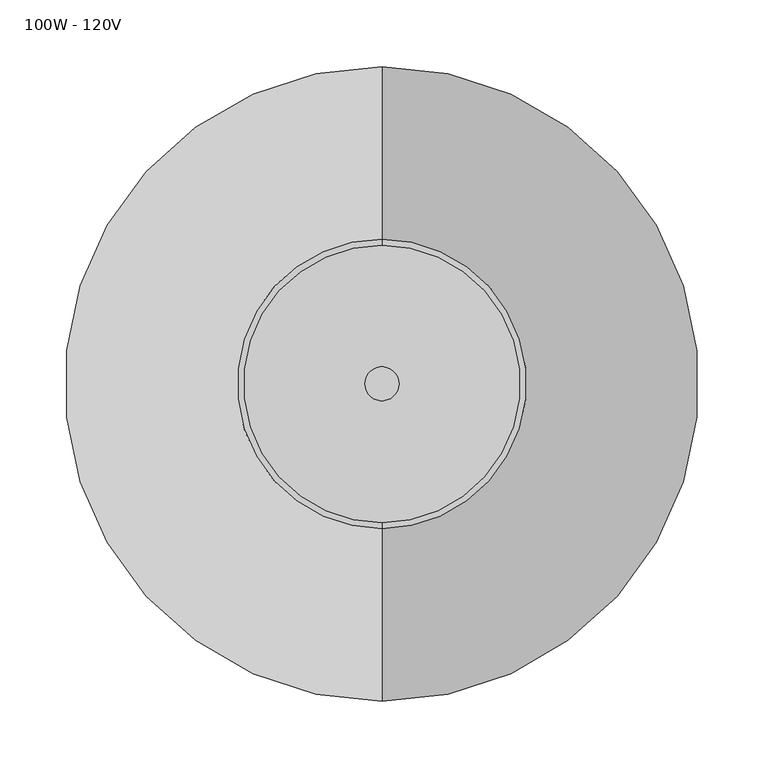
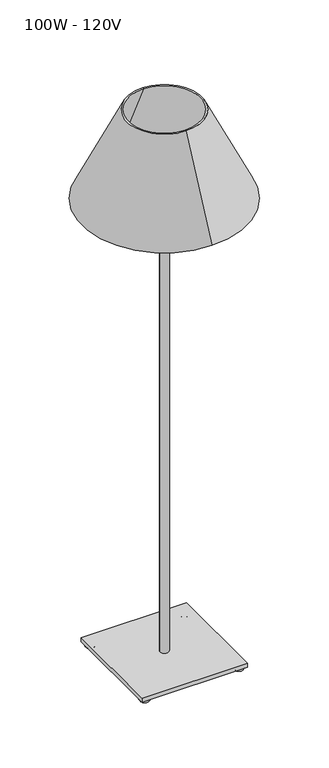
"""IFC4 building model written with IfcOpenShell, lengths in millimetres: light fixture geometry, 100W - 120V."""

from ifc_helpers import new_model, si_unit, point, frame, origin, origin_2d, place, context, project, spatial, polyline, circle_curve, ellipse_curve, trimmed, segment, composite_curve, outline, extrude, source, transform, mapped, element, save
from ifc_brep_helpers import plane_surface, revolved_surface, advanced_brep


def light_fixture_100w_120v_8564026f(model_context):
    return source(origin(), model_context, "Body", "SolidModel", [
        extrude(outline(composite_curve([segment(trimmed(circle_curve(origin_2d(), 12.7), [point((-12.7, 0.0))], [point((12.7, 0.0))], False, "CARTESIAN"), True, "CONTINUOUS"), segment(trimmed(circle_curve(origin_2d(), 12.7), [point((12.7, 0.0))], [point((-12.7, 0.0))], False, "CARTESIAN"), True, "CONTINUOUS")], self_intersect=False)), frame((0.0, 0.0, 24.9639672), z_axis=(0.0, 0.0, 1.0), x_axis=(1.0, 0.0, 0.0)), (0.0, 0.0, 1.0), 1499.0360328),
        extrude(outline(polyline([(152.4, 152.4), (152.4, -152.4), (-152.4, -152.4), (-152.4, 152.4), (152.4, 152.4)])), frame((0.0, 0.0, 12.6871384), z_axis=(0.0, 0.0, 1.0), x_axis=(1.0, 0.0, 0.0)), (0.0, 0.0, 1.0), 12.2768288),
        advanced_brep(
        [(133.9366871, -135.595774, 0.0), (140.1544999, -135.595774, 0.0), (140.1544999, -135.595774, 12.6871384), (133.9366871, -135.595774, 12.6871384), (121.2495488, -135.595774, 12.6871384), (152.8416383, -135.595774, 12.6871384)],
        [
            (0, 1, circle_curve(frame((137.0455935, -135.595774, 0.0), z_axis=(0.0, 0.0, -1.0), x_axis=(0.0, 1.0, 0.0)), 3.1089064)),
            (1, 2),
            (2, 3, circle_curve(frame((137.0455935, -135.595774, 12.6871384), z_axis=(0.0, 0.0, 1.0), x_axis=(0.0, 1.0, 0.0)), 3.1089064)),
            (3, 0),
            (1, 0, circle_curve(frame((137.0455935, -135.595774, 0.0), z_axis=(0.0, 0.0, -1.0), x_axis=(0.0, 1.0, 0.0)), 3.1089064)),
            (3, 2, circle_curve(frame((137.0455935, -135.595774, 12.6871384), z_axis=(0.0, 0.0, 1.0), x_axis=(0.0, 1.0, 0.0)), 3.1089064)),
            (4, 5, circle_curve(frame((137.0455935, -135.595774, 12.6871384), z_axis=(0.0, 0.0, -1.0), x_axis=(0.0, 1.0, 0.0)), 15.7960447)),
            (5, 1, circle_curve(frame((140.1544999, -135.595774, 12.6871384), z_axis=(0.0, 1.0, 0.0), x_axis=(1.0, 0.0, 0.0)), 12.6871384)),
            (0, 4, circle_curve(frame((133.9366871, -135.595774, 12.6871384), z_axis=(0.0, 1.0, 0.0), x_axis=(-1.0, 0.0, 0.0)), 12.6871384)),
            (5, 4, circle_curve(frame((137.0455935, -135.595774, 12.6871384), z_axis=(0.0, 0.0, -1.0), x_axis=(0.0, 1.0, 0.0)), 15.7960447)),
            (2, 5),
            (4, 3),
        ],
        [
            revolved_surface(polyline([(137.0455935, -132.4868676, 12.6871384), (137.0455935, -132.4868676, 0.0)]), (137.0455935, -135.595774, 0.0), (0.0, 0.0, 1.0)),
            revolved_surface(trimmed(ellipse_curve(frame((137.0455935, -132.4868676, 12.6871384), z_axis=(1.0, 0.0, 0.0), x_axis=(0.0, 1.0, 0.0)), 12.6871384, 12.6871384), [point((137.0455935, -132.4868676, 0.0))], [point((137.0455935, -119.7997292, 12.6871384))], True, "CARTESIAN"), (137.0455935, -135.595774, 0.0), (0.0, 0.0, 1.0)),
            plane_surface(frame((137.0455935, -135.595774, 12.6871384), z_axis=(0.0, 0.0, 1.0), x_axis=(0.0, 1.0, 0.0))),
        ],
        [
            (0, [[1, 2, 3, 4]]),
            (0, [[5, -4, 6, -2]]),
            (1, [[7, 8, -1, 9]]),
            (1, [[10, -9, -5, -8]]),
            (2, [[-3, 11, -7, 12]]),
            (2, [[-6, -12, -10, -11]]),
        ],
    ),
        advanced_brep(
        [(-138.5460372, -136.1907144, 0.0), (-132.3282244, -136.1907144, 0.0), (-132.3282244, -136.1907144, 12.6871384), (-138.5460372, -136.1907144, 12.6871384), (-151.2331755, -136.1907144, 12.6871384), (-119.641086, -136.1907144, 12.6871384)],
        [
            (0, 1, circle_curve(frame((-135.4371308, -136.1907144, 0.0), z_axis=(0.0, 0.0, -1.0), x_axis=(0.0, 1.0, 0.0)), 3.1089064)),
            (1, 2),
            (2, 3, circle_curve(frame((-135.4371308, -136.1907144, 12.6871384), z_axis=(0.0, 0.0, 1.0), x_axis=(0.0, 1.0, 0.0)), 3.1089064)),
            (3, 0),
            (1, 0, circle_curve(frame((-135.4371308, -136.1907144, 0.0), z_axis=(0.0, 0.0, -1.0), x_axis=(0.0, 1.0, 0.0)), 3.1089064)),
            (3, 2, circle_curve(frame((-135.4371308, -136.1907144, 12.6871384), z_axis=(0.0, 0.0, 1.0), x_axis=(0.0, 1.0, 0.0)), 3.1089064)),
            (4, 5, circle_curve(frame((-135.4371308, -136.1907144, 12.6871384), z_axis=(0.0, 0.0, -1.0), x_axis=(0.0, 1.0, 0.0)), 15.7960447)),
            (5, 1, circle_curve(frame((-132.3282244, -136.1907144, 12.6871384), z_axis=(0.0, 1.0, 0.0), x_axis=(1.0, 0.0, 0.0)), 12.6871384)),
            (0, 4, circle_curve(frame((-138.5460372, -136.1907144, 12.6871384), z_axis=(0.0, 1.0, 0.0), x_axis=(-1.0, 0.0, 0.0)), 12.6871384)),
            (5, 4, circle_curve(frame((-135.4371308, -136.1907144, 12.6871384), z_axis=(0.0, 0.0, -1.0), x_axis=(0.0, 1.0, 0.0)), 15.7960447)),
            (2, 5),
            (4, 3),
        ],
        [
            revolved_surface(polyline([(-135.4371308, -133.081808, 12.6871384), (-135.4371308, -133.081808, 0.0)]), (-135.4371308, -136.1907144, 0.0), (0.0, 0.0, 1.0)),
            revolved_surface(trimmed(ellipse_curve(frame((-135.4371308, -133.081808, 12.6871384), z_axis=(1.0, 0.0, 0.0), x_axis=(0.0, 1.0, 0.0)), 12.6871384, 12.6871384), [point((-135.4371308, -133.081808, 0.0))], [point((-135.4371308, -120.3946697, 12.6871384))], True, "CARTESIAN"), (-135.4371308, -136.1907144, 0.0), (0.0, 0.0, 1.0)),
            plane_surface(frame((-135.4371308, -136.1907144, 12.6871384), z_axis=(0.0, 0.0, 1.0), x_axis=(0.0, 1.0, 0.0))),
        ],
        [
            (0, [[1, 2, 3, 4]]),
            (0, [[5, -4, 6, -2]]),
            (1, [[7, 8, -1, 9]]),
            (1, [[10, -9, -5, -8]]),
            (2, [[-3, 11, -7, 12]]),
            (2, [[-6, -12, -10, -11]]),
        ],
    ),
        advanced_brep(
        [(-139.1409776, 135.6970694, 0.0), (-132.9231648, 135.6970694, 0.0), (-132.9231648, 135.6970694, 12.6871384), (-139.1409776, 135.6970694, 12.6871384), (-151.828116, 135.6970694, 12.6871384), (-120.2360265, 135.6970694, 12.6871384)],
        [
            (0, 1, circle_curve(frame((-136.0320712, 135.6970694, 0.0), z_axis=(0.0, 0.0, -1.0), x_axis=(0.0, 1.0, 0.0)), 3.1089064)),
            (1, 2),
            (2, 3, circle_curve(frame((-136.0320712, 135.6970694, 12.6871384), z_axis=(0.0, 0.0, 1.0), x_axis=(0.0, 1.0, 0.0)), 3.1089064)),
            (3, 0),
            (1, 0, circle_curve(frame((-136.0320712, 135.6970694, 0.0), z_axis=(0.0, 0.0, -1.0), x_axis=(0.0, 1.0, 0.0)), 3.1089064)),
            (3, 2, circle_curve(frame((-136.0320712, 135.6970694, 12.6871384), z_axis=(0.0, 0.0, 1.0), x_axis=(0.0, 1.0, 0.0)), 3.1089064)),
            (4, 5, circle_curve(frame((-136.0320712, 135.6970694, 12.6871384), z_axis=(0.0, 0.0, -1.0), x_axis=(0.0, 1.0, 0.0)), 15.7960447)),
            (5, 1, circle_curve(frame((-132.9231648, 135.6970694, 12.6871384), z_axis=(0.0, 1.0, 0.0), x_axis=(1.0, 0.0, 0.0)), 12.6871384)),
            (0, 4, circle_curve(frame((-139.1409776, 135.6970694, 12.6871384), z_axis=(0.0, 1.0, 0.0), x_axis=(-1.0, 0.0, 0.0)), 12.6871384)),
            (5, 4, circle_curve(frame((-136.0320712, 135.6970694, 12.6871384), z_axis=(0.0, 0.0, -1.0), x_axis=(0.0, 1.0, 0.0)), 15.7960447)),
            (2, 5),
            (4, 3),
        ],
        [
            revolved_surface(polyline([(-136.0320712, 138.8059758, 12.6871384), (-136.0320712, 138.8059758, 0.0)]), (-136.0320712, 135.6970694, 0.0), (0.0, 0.0, 1.0)),
            revolved_surface(trimmed(ellipse_curve(frame((-136.0320712, 138.8059758, 12.6871384), z_axis=(1.0, 0.0, 0.0), x_axis=(0.0, 1.0, 0.0)), 12.6871384, 12.6871384), [point((-136.0320712, 138.8059758, 0.0))], [point((-136.0320712, 151.4931142, 12.6871384))], True, "CARTESIAN"), (-136.0320712, 135.6970694, 0.0), (0.0, 0.0, 1.0)),
            plane_surface(frame((-136.0320712, 135.6970694, 12.6871384), z_axis=(0.0, 0.0, 1.0), x_axis=(0.0, 1.0, 0.0))),
        ],
        [
            (0, [[1, 2, 3, 4]]),
            (0, [[5, -4, 6, -2]]),
            (1, [[7, 8, -1, 9]]),
            (1, [[10, -9, -5, -8]]),
            (2, [[-3, 11, -7, 12]]),
            (2, [[-6, -12, -10, -11]]),
        ],
    ),
        advanced_brep(
        [(133.2106985, 136.0573029, 0.0), (139.4285113, 136.0573029, 0.0), (139.4285113, 136.0573029, 12.6871384), (133.2106985, 136.0573029, 12.6871384), (120.5235602, 136.0573029, 12.6871384), (152.1156497, 136.0573029, 12.6871384)],
        [
            (0, 1, circle_curve(frame((136.3196049, 136.0573029, 0.0), z_axis=(0.0, 0.0, -1.0), x_axis=(0.0, 1.0, 0.0)), 3.1089064)),
            (1, 2),
            (2, 3, circle_curve(frame((136.3196049, 136.0573029, 12.6871384), z_axis=(0.0, 0.0, 1.0), x_axis=(0.0, 1.0, 0.0)), 3.1089064)),
            (3, 0),
            (1, 0, circle_curve(frame((136.3196049, 136.0573029, 0.0), z_axis=(0.0, 0.0, -1.0), x_axis=(0.0, 1.0, 0.0)), 3.1089064)),
            (3, 2, circle_curve(frame((136.3196049, 136.0573029, 12.6871384), z_axis=(0.0, 0.0, 1.0), x_axis=(0.0, 1.0, 0.0)), 3.1089064)),
            (4, 5, circle_curve(frame((136.3196049, 136.0573029, 12.6871384), z_axis=(0.0, 0.0, -1.0), x_axis=(0.0, 1.0, 0.0)), 15.7960447)),
            (5, 1, circle_curve(frame((139.4285113, 136.0573029, 12.6871384), z_axis=(0.0, 1.0, 0.0), x_axis=(1.0, 0.0, 0.0)), 12.6871384)),
            (0, 4, circle_curve(frame((133.2106985, 136.0573029, 12.6871384), z_axis=(0.0, 1.0, 0.0), x_axis=(-1.0, 0.0, 0.0)), 12.6871384)),
            (5, 4, circle_curve(frame((136.3196049, 136.0573029, 12.6871384), z_axis=(0.0, 0.0, -1.0), x_axis=(0.0, 1.0, 0.0)), 15.7960447)),
            (2, 5),
            (4, 3),
        ],
        [
            revolved_surface(polyline([(136.3196049, 139.1662093, 12.6871384), (136.3196049, 139.1662093, 0.0)]), (136.3196049, 136.0573029, 0.0), (0.0, 0.0, 1.0)),
            revolved_surface(trimmed(ellipse_curve(frame((136.3196049, 139.1662093, 12.6871384), z_axis=(1.0, 0.0, 0.0), x_axis=(0.0, 1.0, 0.0)), 12.6871384, 12.6871384), [point((136.3196049, 139.1662093, 0.0))], [point((136.3196049, 151.8533477, 12.6871384))], True, "CARTESIAN"), (136.3196049, 136.0573029, 0.0), (0.0, 0.0, 1.0)),
            plane_surface(frame((136.3196049, 136.0573029, 12.6871384), z_axis=(0.0, 0.0, 1.0), x_axis=(0.0, 1.0, 0.0))),
        ],
        [
            (0, [[1, 2, 3, 4]]),
            (0, [[5, -4, 6, -2]]),
            (1, [[7, 8, -1, 9]]),
            (1, [[10, -9, -5, -8]]),
            (2, [[-3, 11, -7, 12]]),
            (2, [[-6, -12, -10, -11]]),
        ],
    ),
        advanced_brep(
        [(0.0, -233.3382251, 1403.5752564), (0.0, 233.3382251, 1403.5752564), (0.0, 104.0586089, 1674.1859784), (0.0, -104.0586089, 1674.1859784), (0.0, -237.8523754, 1403.5752564), (0.0, 237.8523754, 1403.5752564), (0.0, -108.5727592, 1674.1859784), (0.0, 108.5727592, 1674.1859784)],
        [
            (0, 1, circle_curve(frame((0.0, 0.0, 1403.5752564), z_axis=(0.0, 0.0, -1.0), x_axis=(0.0, 1.0, 0.0)), 233.3382251)),
            (1, 2),
            (2, 3, circle_curve(frame((0.0, 0.0, 1674.1859784), z_axis=(0.0, 0.0, 1.0), x_axis=(0.0, 1.0, 0.0)), 104.0586089)),
            (3, 0),
            (1, 0, circle_curve(frame((0.0, 0.0, 1403.5752564), z_axis=(0.0, 0.0, -1.0), x_axis=(0.0, 1.0, 0.0)), 233.3382251)),
            (3, 2, circle_curve(frame((0.0, 0.0, 1674.1859784), z_axis=(0.0, 0.0, 1.0), x_axis=(0.0, 1.0, 0.0)), 104.0586089)),
            (4, 5, circle_curve(frame((0.0, 0.0, 1403.5752564), z_axis=(0.0, 0.0, -1.0), x_axis=(0.0, 1.0, 0.0)), 237.8523754)),
            (5, 1),
            (0, 4),
            (5, 4, circle_curve(frame((0.0, 0.0, 1403.5752564), z_axis=(0.0, 0.0, -1.0), x_axis=(0.0, 1.0, 0.0)), 237.8523754)),
            (6, 7, circle_curve(frame((0.0, 0.0, 1674.1859784), z_axis=(0.0, 0.0, -1.0), x_axis=(0.0, 1.0, 0.0)), 108.5727592)),
            (7, 5),
            (4, 6),
            (7, 6, circle_curve(frame((0.0, 0.0, 1674.1859784), z_axis=(0.0, 0.0, -1.0), x_axis=(0.0, 1.0, 0.0)), 108.5727592)),
            (2, 7),
            (6, 3),
        ],
        [
            revolved_surface(polyline([(0.0, 104.0586089, 1674.1859784), (0.0, 233.3382251, 1403.5752564)]), (0.0, 0.0, 1713.8233367), (0.0, 0.0, 1.0)),
            plane_surface(frame((0.0, 0.0, 1403.5752564), z_axis=(0.0, 0.0, -1.0), x_axis=(0.0, 1.0, 0.0))),
            revolved_surface(polyline([(0.0, 237.8523754, 1403.5752564), (0.0, 108.5727592, 1674.1859784)]), (0.0, 0.0, 1713.8233367), (0.0, 0.0, 1.0)),
            plane_surface(frame((0.0, 0.0, 1674.1859784), z_axis=(0.0, 0.0, 1.0), x_axis=(0.0, 1.0, 0.0))),
        ],
        [
            (0, [[1, 2, 3, 4]]),
            (0, [[5, -4, 6, -2]]),
            (1, [[7, 8, -1, 9]]),
            (1, [[10, -9, -5, -8]]),
            (2, [[11, 12, -7, 13]]),
            (2, [[14, -13, -10, -12]]),
            (3, [[-3, 15, -11, 16]]),
            (3, [[-6, -16, -14, -15]]),
        ],
    ),
    ])


if __name__ == "__main__":
    model = new_model("IFC4")
    model_context = context("Model", 3, world=origin())
    ifc_project = project(units=[si_unit("LENGTHUNIT", "METRE", prefix="MILLI")], contexts=[model_context])
    site = spatial("IfcSite", under=ifc_project)
    building = spatial("IfcBuilding", under=site)
    placement = place(None, origin())
    light_fixture_100w_120v_shape = light_fixture_100w_120v_8564026f(model_context)
    element("IfcLightFixture", 1, ObjectType="100W - 120V", at=placement, inside=building, context=model_context, shape_type="MappedRepresentation", body=[
        mapped(light_fixture_100w_120v_shape, transform((0.0, 0.0, 0.0), x_axis=(1.0, 0.0, 0.0), y_axis=(0.0, 1.0, 0.0), z_axis=(0.0, 0.0, 1.0))),
    ])
    save(model, "model.ifc")

# Revit data of these elements
# Type "100W - 120V"
#   Assembly Code = "D5020220"
#   Lamp = "A-19"
#   Wattage Comments = "100"
#   Wattage = 100 W
#   built-in parameter 1150110 = 1 (stored number, unit not read)
#   built-in parameter 1114217 = 1 (stored number, unit not read)
#   built-in parameter 1150109 = 1 (stored number, unit not read)
#   built-in parameter 1150113 = 1 (stored number, unit not read)
#   built-in parameter 1150115 = 1 (stored number, unit not read)
#   built-in parameter 1150105 = 139.261 (stored number, unit not read)
#   Light Source Symbol Size = 2' - 0"
#   built-in parameter 1150112 = 1 (stored number, unit not read)
#   built-in parameter 1150114 = 1 (stored number, unit not read)
#   built-in parameter 1150107 = 2800 (stored number, unit not read)
#   built-in parameter 1150106 = 1.39261 (stored number, unit not read)
#   built-in parameter 1150104 = 1.6258 (stored number, unit not read)
#   Ballast Voltage = 120 V
#   built-in parameter 1114218 = 1 (stored number, unit not read)
#   built-in parameter 1150133 = 10 (stored number, unit not read)
#   Lumens = 1750 lm
#   Apparent Load = 100 VA
#   built-in parameter 1150134 = 4
#   built-in parameter 1150137 = 1
#   Color Filter = 16777215
#   Ballast Number of Poles = 1
#   Shade = Glass, Frosted
#   Stand = Steel, Chrome Plated
#   Dimming Lamp Color Temperature Shift = (empty or 0)
# Element 1 (IfcLightFixture, "100W - 120V")
#   Materials on its faces: "Steel, Chrome Plated", "Glass, Frosted"
# Materials
#   "Glass, Frosted": class "Glass", colour RGB 250 244 225, transparency 0.55, Description = "physical material", Cost = 0
#   "Steel, Chrome Plated": class "Metal", colour RGB 17 17 17, transparency 0, Description = "Chromiuim plated steel", Cost = 0
